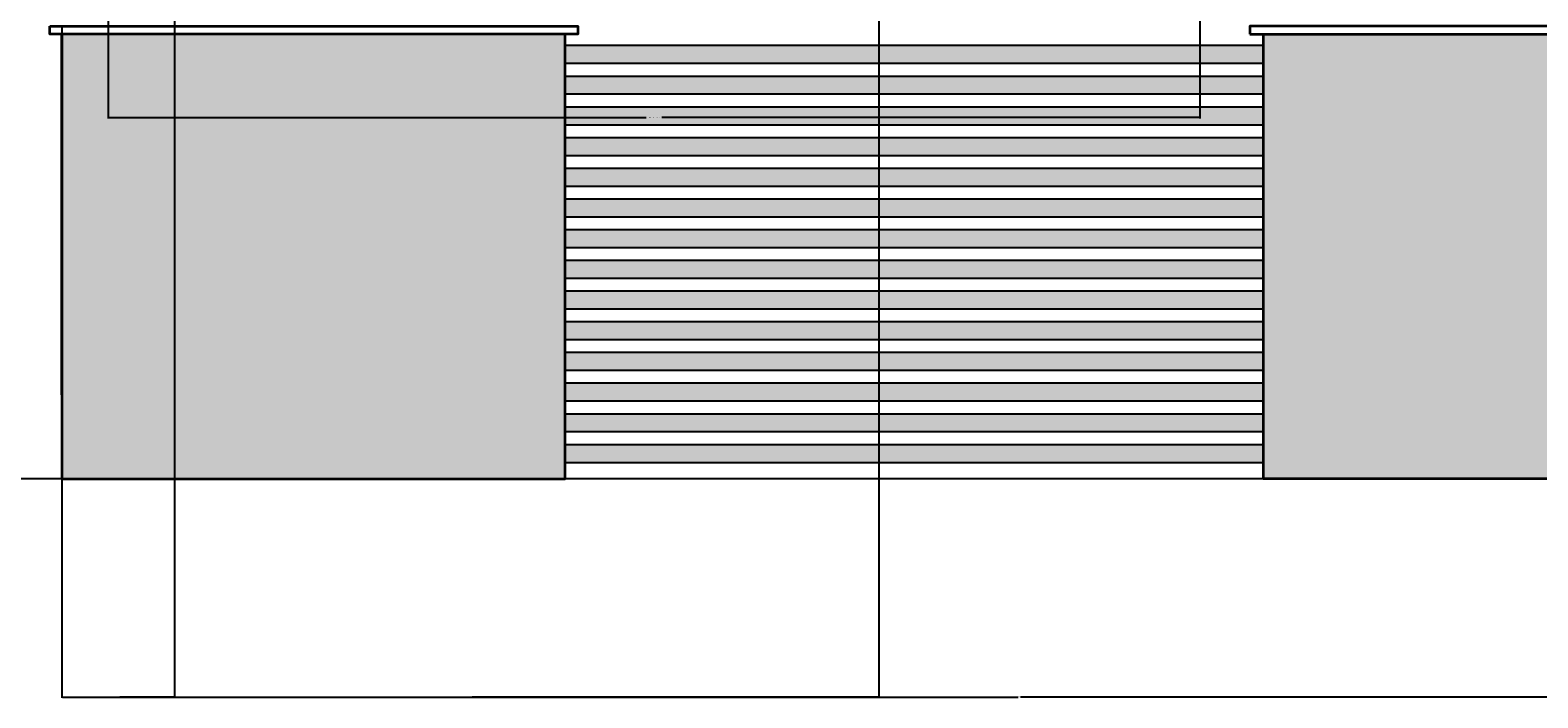
# Model space of a CAD drawing. Units: feet. Extents: x 1141 to 2858, y 751 to 1654.
# Tile 2 of 13: x 1718 to 2096, y 751 to 918. Entities that reach past the tile are written whole.
import ezdxf

# ---------------------------------------------------------------- set-up
doc = ezdxf.new("R2010")
doc.units = ezdxf.units.FT
for name, color, linetype, lineweight in [('A-ANNO-DIMS', 2, 'Continuous', 18), ('A-DOOR', 3, 'Continuous', 25), ('A-ELEV', 7, 'Continuous', 35), ('A-ELEV-PATT', 8, 'Continuous', 13)]:
    doc.layers.add(name, color=color, linetype=linetype, lineweight=lineweight)
doc.styles.get("Standard").update_dxf_attribs({"font": 'arial.ttf'})
doc.dimstyles.get("Standard").update_dxf_attribs({"dimtxt": 0.18, "dimasz": 0.18, "dimexe": 0.18, "dimexo": 0.0625, "dimgap": 0.09, "dimtad": 0, "dimtih": 1, "dimtoh": 1, "dimdec": 1, "dimzin": 0, "dimdsep": 46, "dimlunit": 3, "dimtxsty": 'Standard', "dimcen": 0.09, "dimadec": 0, "dimazin": 0, "dimtfac": 1, "dimtdec": 1, "dimtofl": 0, "dimtmove": 0, "dimatfit": 3, "dimfxl": 1, "dimtolj": 1, "dimtzin": 0, "dimarcsym": 0})

# ---------------------------------------------------------------- blocks, each defined once
blk = doc.blocks.new('*D18')
at = {"layer": 'A-ANNO-DIMS', "color": 0, "lineweight": -2, "transparency": 16777216}
for p, q in [((1737.61, 937.42), (1737.61, 896.25)), ((2011.29, 937.42), (2011.29, 896.25)), ((1737.79, 896.43), (1872.51, 896.43)), ((2011.11, 896.43), (1876.38, 896.43))]:
    blk.add_line(p, q, dxfattribs=at)
at = {"layer": 'A-ANNO-DIMS', "color": 0, "transparency": 16777216}
for points in [[(1737.79, 896.46), (1737.79, 896.4), (1737.61, 896.43)], [(2011.11, 896.46), (2011.11, 896.4), (2011.29, 896.43)]]:
    blk.add_solid(points, dxfattribs=at)
at = {"layer": 'Defpoints', "color": 0, "transparency": 16777216}
for p in [(1737.61, 937.48), (2011.29, 937.48), (2011.29, 896.43)]:
    blk.add_point(p, dxfattribs=at)
at = {"layer": 'A-ANNO-DIMS', "color": 0, "transparency": 16777216, "insert": (1874.45, 896.43), "char_height": 0.18, "attachment_point": 5}
blk.add_mtext('\\A1;BALCONY GLAZING A 274 TYP.', dxfattribs=at)
blk = doc.blocks.new('*D22')
at = {"layer": 'A-ANNO-DIMS', "color": 0, "lineweight": -2, "transparency": 16777216}
for p, q in [((1726.03, 805.84), (1726.03, 751.07)), ((2206.03, 805.84), (2206.03, 751.07)), ((1726.21, 751.25), (1965.74, 751.25)), ((2205.85, 751.25), (1966.32, 751.25))]:
    blk.add_line(p, q, dxfattribs=at)
at = {"layer": 'A-ANNO-DIMS', "color": 0, "transparency": 16777216}
for points in [[(1726.21, 751.28), (1726.21, 751.22), (1726.03, 751.25)], [(2205.85, 751.28), (2205.85, 751.22), (2206.03, 751.25)]]:
    blk.add_solid(points, dxfattribs=at)
at = {"layer": 'Defpoints', "color": 0, "transparency": 16777216}
for p in [(1726.03, 805.9), (2206.03, 805.9), (2206.03, 751.25)]:
    blk.add_point(p, dxfattribs=at)
at = {"layer": 'A-ANNO-DIMS', "color": 0, "transparency": 16777216, "insert": (1966.03, 751.25), "char_height": 0.18, "attachment_point": 5}
blk.add_mtext('\\A1;480', dxfattribs=at)
blk = doc.blocks.new('*D24')
at = {"layer": 'A-ANNO-DIMS', "color": 0, "lineweight": -2, "transparency": 16777216}
for p, q in [((1725.97, 1599.45), (1668.14, 1599.45)), ((1668.32, 1599.27), (1668.32, 1202.86)), ((1668.32, 806.08), (1668.32, 1202.49)), ((1725.97, 805.9), (1668.14, 805.9))]:
    blk.add_line(p, q, dxfattribs=at)
at = {"layer": 'A-ANNO-DIMS', "color": 0, "transparency": 16777216}
for points in [[(1668.29, 1599.27), (1668.35, 1599.27), (1668.32, 1599.45)], [(1668.29, 806.08), (1668.35, 806.08), (1668.32, 805.9)]]:
    blk.add_solid(points, dxfattribs=at)
at = {"layer": 'Defpoints', "color": 0, "transparency": 16777216}
for p in [(1668.32, 1599.45), (1726.03, 1599.45), (1726.03, 805.9)]:
    blk.add_point(p, dxfattribs=at)
at = {"layer": 'A-ANNO-DIMS', "color": 0, "transparency": 16777216, "insert": (1668.32, 1202.68), "char_height": 0.18, "attachment_point": 5}
blk.add_mtext('\\A1;793.6', dxfattribs=at)
blk = doc.blocks.new('*D39')
at = {"layer": 'A-ANNO-DIMS', "color": 0, "lineweight": -2, "transparency": 16777216}
for p, q in [((2319.24, 1599.45), (1668.14, 1599.45)), ((1668.32, 1599.27), (1668.32, 1202.86)), ((1668.32, 806.08), (1668.32, 1202.49)), ((2319.24, 805.9), (1668.14, 805.9))]:
    blk.add_line(p, q, dxfattribs=at)
at = {"layer": 'A-ANNO-DIMS', "color": 0, "transparency": 16777216}
for points in [[(1668.29, 1599.27), (1668.35, 1599.27), (1668.32, 1599.45)], [(1668.29, 806.08), (1668.35, 806.08), (1668.32, 805.9)]]:
    blk.add_solid(points, dxfattribs=at)
at = {"layer": 'Defpoints', "color": 0, "transparency": 16777216}
for p in [(1668.32, 1599.45), (2319.3, 1599.45), (2319.3, 805.9)]:
    blk.add_point(p, dxfattribs=at)
at = {"layer": 'A-ANNO-DIMS', "color": 0, "transparency": 16777216, "insert": (1668.32, 1202.68), "char_height": 0.18, "attachment_point": 5}
blk.add_mtext('\\A1;793.6', dxfattribs=at)
blk = doc.blocks.new('*D89')
at = {"layer": 'A-ANNO-DIMS', "color": 0, "lineweight": -2, "transparency": 16777216}
for p, q in [((1754.24, 946.71), (1754.24, 751.07)), ((1726.03, 919.28), (1726.03, 751.07)), ((1726.21, 751.25), (1739.76, 751.25)), ((1754.06, 751.25), (1740.52, 751.25))]:
    blk.add_line(p, q, dxfattribs=at)
at = {"layer": 'A-ANNO-DIMS', "color": 0, "transparency": 16777216}
for points in [[(1726.21, 751.28), (1726.21, 751.22), (1726.03, 751.25)], [(1754.06, 751.28), (1754.06, 751.22), (1754.24, 751.25)]]:
    blk.add_solid(points, dxfattribs=at)
at = {"layer": 'Defpoints', "color": 0, "transparency": 16777216}
for p in [(1754.24, 946.77), (1726.03, 919.34), (1754.24, 751.25)]:
    blk.add_point(p, dxfattribs=at)
at = {"layer": 'A-ANNO-DIMS', "color": 0, "transparency": 16777216, "insert": (1740.14, 751.25), "char_height": 0.18, "attachment_point": 5}
blk.add_mtext('\\A1;28.21', dxfattribs=at)
blk = doc.blocks.new('*D90')
at = {"layer": 'A-ANNO-DIMS', "color": 0, "lineweight": -2, "transparency": 16777216}
for p, q in [((1930.8, 951.37), (1930.8, 751.07)), ((1726.03, 919.28), (1726.03, 751.07)), ((1726.21, 751.25), (1827.95, 751.25)), ((1930.62, 751.25), (1828.88, 751.25))]:
    blk.add_line(p, q, dxfattribs=at)
at = {"layer": 'A-ANNO-DIMS', "color": 0, "transparency": 16777216}
for points in [[(1726.21, 751.28), (1726.21, 751.22), (1726.03, 751.25)], [(1930.62, 751.28), (1930.62, 751.22), (1930.8, 751.25)]]:
    blk.add_solid(points, dxfattribs=at)
at = {"layer": 'Defpoints', "color": 0, "transparency": 16777216}
for p in [(1930.8, 951.43), (1726.03, 919.34), (1930.8, 751.25)]:
    blk.add_point(p, dxfattribs=at)
at = {"layer": 'A-ANNO-DIMS', "color": 0, "transparency": 16777216, "insert": (1828.42, 751.25), "char_height": 0.18, "attachment_point": 5}
blk.add_mtext('\\A1;204.77', dxfattribs=at)

msp = doc.modelspace()

# ---------------------------------------------------------------- hatches: boundary and pattern name
at = {"layer": 'A-ELEV-PATT'}
h = msp.add_hatch(color=256, dxfattribs=at)
h.dxf.hatch_style = 1
h.paths.add_polyline_path([(2206.032, 1599.4527), (2192.689, 1599.4527), (2192.689, 919.339), (2206.032, 919.339)])
h.paths.add_polyline_path([(2190.2416, 1599.4527), (2175.463, 1599.4527), (2175.463, 919.339), (2190.2416, 919.339)])
h.paths.add_polyline_path([(2173.0156, 1599.4527), (2117.407, 1599.4527), (2117.407, 919.339), (2173.0156, 919.339)])
h.paths.add_polyline_path([(2022.8666, 1057.9008), (1726.032, 1057.9008), (1726.032, 925.9008), (2022.8666, 925.9008)])
h.paths.add_polyline_path([(1737.6123, 937.4811), (1737.6123, 1046.3205), (2011.2863, 1046.3205), (2011.2863, 937.4811)], flags=16)
h.paths.add_polyline_path([(1754.2423, 946.7736), (1754.2423, 1033.2183), (2004.2323, 1033.2183), (2004.2323, 946.7736), (2004.3069, 946.6754), (1906.0824, 946.6754)], flags=0)
h.paths.add_polyline_path([(1900.5421, 946.7736), (1857.5566, 946.7736), (1857.5566, 1033.2183), (1900.5421, 1033.2183)], flags=0)
h.paths.add_polyline_path([(1910.8368, 951.4297), (1910.8368, 1022.7957), (1999.478, 1022.7957), (1999.478, 951.4297)], flags=0)
h.paths.add_polyline_path([(1930.8039, 951.4297), (1930.8039, 1022.7957), (1932.373, 1022.7957), (1932.373, 951.4297)], flags=0)
h.paths.add_polyline_path([(1851.6414, 946.7736), (1826.5664, 946.7736), (1826.5664, 967.8234), (1793.4402, 967.8234), (1793.4402, 946.7736), (1790.4043, 946.7736), (1790.4043, 967.8234), (1754.2423, 967.8234), (1754.2423, 970.4796), (1790.4043, 970.4796), (1790.4043, 1033.2183), (1793.4402, 1033.2183), (1793.4402, 970.4796), (1826.5664, 970.4796), (1826.5664, 1033.2183), (1851.6414, 1033.2183)], flags=0)
h.paths.add_polyline_path([(1954.3728, 951.4297), (1954.3728, 1022.7957), (1955.9419, 1022.7957), (1955.9419, 951.4297)], flags=0)
h.paths.add_polyline_path([(1977.7327, 951.4297), (1977.7327, 1022.7957), (1979.3018, 1022.7957), (1979.3018, 951.4297)], flags=0)
h.paths.add_polyline_path([(2022.8666, 1193.2888), (1726.032, 1193.2888), (1726.032, 1061.2888), (2022.8666, 1061.2888)])
h.paths.add_polyline_path([(1737.6123, 1072.869), (1737.6123, 1181.7085), (2011.2863, 1181.7085), (2011.2863, 1072.869)], flags=16)
h.paths.add_polyline_path([(1754.2423, 1082.1616), (1754.2423, 1168.6063), (2004.2323, 1168.6063), (2004.2323, 1082.1616), (2004.3069, 1082.0634), (1906.0824, 1082.0634)], flags=0)
h.paths.add_polyline_path([(1900.5421, 1082.1616), (1857.5566, 1082.1616), (1857.5566, 1168.6063), (1900.5421, 1168.6063)], flags=0)
h.paths.add_polyline_path([(1910.8368, 1086.8177), (1910.8368, 1158.1837), (1999.478, 1158.1837), (1999.478, 1086.8177)], flags=0)
h.paths.add_polyline_path([(1930.8039, 1086.8177), (1930.8039, 1158.1837), (1932.373, 1158.1837), (1932.373, 1086.8177)], flags=0)
h.paths.add_polyline_path([(1851.6414, 1082.1616), (1826.5664, 1082.1616), (1826.5664, 1103.2114), (1793.4402, 1103.2114), (1793.4402, 1082.1616), (1790.4043, 1082.1616), (1790.4043, 1103.2114), (1754.2423, 1103.2114), (1754.2423, 1105.8676), (1790.4043, 1105.8676), (1790.4043, 1168.6063), (1793.4402, 1168.6063), (1793.4402, 1105.8676), (1826.5664, 1105.8676), (1826.5664, 1168.6063), (1851.6414, 1168.6063)], flags=0)
h.paths.add_polyline_path([(1954.3728, 1086.8177), (1954.3728, 1158.1837), (1955.9419, 1158.1837), (1955.9419, 1086.8177)], flags=0)
h.paths.add_polyline_path([(1977.7327, 1086.8177), (1977.7327, 1158.1837), (1979.3018, 1158.1837), (1979.3018, 1086.8177)], flags=0)
h.paths.add_polyline_path([(2022.8666, 1599.4527), (1726.032, 1599.4527), (1726.032, 1467.4527), (2022.8666, 1467.4527)])
h.paths.add_polyline_path([(2011.2863, 1479.033), (1737.6123, 1479.033), (1737.6123, 1587.8725), (2011.2863, 1587.8725)], flags=16)
h.paths.add_polyline_path([(2004.2323, 1488.3255), (1754.2423, 1488.3255), (1754.2423, 1574.7702), (2004.2323, 1574.7702)], flags=0)
h.paths.add_polyline_path([(1829.1345, 1544.6458), (1914.1177, 1544.6458), (1914.1177, 1539.5463), (1830.9097, 1539.5463), (1831.6817, 1537.3286), (1914.1177, 1537.3286), (1914.1177, 1532.2291), (1833.4569, 1532.2291), (1834.229, 1530.0113), (1914.1177, 1530.0113), (1914.1177, 1524.9118), (1836.0042, 1524.9118), (1836.7762, 1522.694), (1914.1177, 1522.694), (1914.1177, 1517.5946), (1838.5514, 1517.5946), (1839.3235, 1515.3768), (1914.1177, 1515.3768), (1914.1177, 1510.2773), (1841.0987, 1510.2773), (1841.8707, 1508.0595), (1914.1177, 1508.0595), (1914.1177, 1502.9601), (1843.6459, 1502.9601), (1844.4179, 1500.7423), (1914.1177, 1500.7423), (1914.1177, 1495.6428), (1846.1931, 1495.6428), (1846.9652, 1493.425), (1914.1177, 1493.425), (1914.1177, 1488.3255), (1848.6593, 1488.3255), (1848.6593, 1488.5583)], flags=0)
h.paths.add_polyline_path([(2117.407, 1464.0647), (1820.5724, 1464.0647), (1820.5724, 1332.0647), (2117.407, 1332.0647)])
h.paths.add_polyline_path([(2105.8267, 1452.4845), (2105.8267, 1343.645), (1832.1527, 1343.645), (1832.1527, 1452.4845)], flags=16)
h.paths.add_polyline_path([(2089.1967, 1439.3822), (2089.1967, 1352.9376), (1937.3566, 1352.9376), (1937.3566, 1352.8393), (1839.1321, 1352.8393), (1839.2067, 1352.9376), (1839.2067, 1439.3822), (1937.3566, 1439.3822)], flags=0)
h.paths.add_polyline_path([(2016.8727, 1439.3822), (2016.8727, 1376.6436), (2049.9988, 1376.6436), (2049.9988, 1439.3822), (2053.0347, 1439.3822), (2053.0347, 1376.6436), (2089.1967, 1376.6436), (2089.1967, 1373.9873), (2053.0347, 1373.9873), (2053.0347, 1352.9376), (2049.9988, 1352.9376), (2049.9988, 1373.9873), (2016.8727, 1373.9873), (2016.8727, 1352.9376), (1991.7976, 1352.9376), (1991.7976, 1439.3822)], flags=0)
h.paths.add_polyline_path([(1985.8824, 1439.3822), (1985.8824, 1352.9376), (1942.8969, 1352.9376), (1942.8969, 1439.3822)], flags=0)
h.paths.add_polyline_path([(1932.6022, 1428.9596), (1932.6022, 1357.5937), (1843.961, 1357.5937), (1843.961, 1428.9596)], flags=0)
h.paths.add_polyline_path([(1912.6351, 1428.9596), (1912.6351, 1357.5937), (1911.066, 1357.5937), (1911.066, 1428.9596)], flags=0)
h.paths.add_polyline_path([(1889.0662, 1428.9596), (1889.0662, 1357.5937), (1887.4971, 1357.5937), (1887.4971, 1428.9596)], flags=0)
h.paths.add_polyline_path([(1865.7063, 1428.9596), (1865.7063, 1357.5937), (1864.1372, 1357.5937), (1864.1372, 1428.9596)], flags=0)
h.paths.add_polyline_path([(2117.407, 1328.6768), (1820.5724, 1328.6768), (1820.5724, 1196.6768), (2117.407, 1196.6768)])
h.paths.add_polyline_path([(2105.8267, 1317.0965), (2105.8267, 1208.257), (1832.1527, 1208.257), (1832.1527, 1317.0965)], flags=16)
h.paths.add_polyline_path([(2089.1967, 1303.9943), (2089.1967, 1217.5496), (1937.3566, 1217.5496), (1937.3566, 1217.4513), (1839.1321, 1217.4513), (1839.2067, 1217.5496), (1839.2067, 1303.9943), (1937.3566, 1303.9943)], flags=0)
h.paths.add_polyline_path([(2016.8727, 1303.9943), (2016.8727, 1241.2556), (2049.9988, 1241.2556), (2049.9988, 1303.9943), (2053.0347, 1303.9943), (2053.0347, 1241.2556), (2089.1967, 1241.2556), (2089.1967, 1238.5993), (2053.0347, 1238.5993), (2053.0347, 1217.5496), (2049.9988, 1217.5496), (2049.9988, 1238.5993), (2016.8727, 1238.5993), (2016.8727, 1217.5496), (1991.7976, 1217.5496), (1991.7976, 1303.9943)], flags=0)
h.paths.add_polyline_path([(1985.8824, 1303.9943), (1985.8824, 1217.5496), (1942.8969, 1217.5496), (1942.8969, 1303.9943)], flags=0)
h.paths.add_polyline_path([(1932.6022, 1293.5716), (1932.6022, 1222.2057), (1843.961, 1222.2057), (1843.961, 1293.5716)], flags=0)
h.paths.add_polyline_path([(1912.6351, 1293.5716), (1912.6351, 1222.2057), (1911.066, 1222.2057), (1911.066, 1293.5716)], flags=0)
h.paths.add_polyline_path([(1889.0662, 1293.5716), (1889.0662, 1222.2057), (1887.4971, 1222.2057), (1887.4971, 1293.5716)], flags=0)
h.paths.add_polyline_path([(1865.7063, 1293.5716), (1865.7063, 1222.2057), (1864.1372, 1222.2057), (1864.1372, 1293.5716)], flags=0)
h.paths.add_polyline_path([(2206.032, 917.3598), (2027.2589, 917.3598), (2027.2589, 805.9008), (2206.032, 805.9008)])
h.paths.add_polyline_path([(1852.1771, 917.3598), (1726.032, 917.3598), (1726.032, 805.9008), (1852.1771, 805.9008)])
h.paths.add_polyline_path([(2063.3101, 1580.3829), (2093.938, 1580.3829), (2093.938, 1513.0494), (2063.3101, 1513.0494)])
h.paths.add_polyline_path([(2063.3101, 1580.3829), (2093.938, 1580.3829), (2093.938, 1513.0494), (2063.3101, 1513.0494)])
h = msp.add_hatch(color=256, dxfattribs=at)
h.dxf.hatch_style = 1
h.paths.add_polyline_path([(2004.2323, 1574.7702), (1754.2423, 1574.7702), (1763.3732, 1548.5407), (1979.2491, 1548.5407), (1979.2491, 1488.3255), (2004.2323, 1488.3255)])
h.paths.add_polyline_path([(1754.2423, 1574.7702), (1754.2423, 1488.3255), (1784.3349, 1488.3255)], flags=17)
h.paths.add_polyline_path([(1768.7403, 1548.5407), (1766.0183, 1548.5407), (1786.98, 1488.3255), (1789.702, 1488.3255)], flags=17)
h.paths.add_polyline_path([(1774.1074, 1548.5407), (1771.3854, 1548.5407), (1792.3471, 1488.3255), (1795.0692, 1488.3255)], flags=17)
h.paths.add_polyline_path([(1779.4746, 1548.5407), (1776.7525, 1548.5407), (1797.7142, 1488.3255), (1800.4363, 1488.3255)], flags=17)
h.paths.add_polyline_path([(1784.8417, 1548.5407), (1782.1197, 1548.5407), (1803.0814, 1488.3255), (1805.8034, 1488.3255)], flags=17)
h.paths.add_polyline_path([(1790.2088, 1548.5407), (1787.4868, 1548.5407), (1808.4485, 1488.3255), (1811.1705, 1488.3255)], flags=17)
h.paths.add_polyline_path([(1795.5759, 1548.5407), (1792.8539, 1548.5407), (1813.8156, 1488.3255), (1816.5376, 1488.3255)], flags=17)
h.paths.add_polyline_path([(1800.9431, 1548.5407), (1798.221, 1548.5407), (1819.1827, 1488.3255), (1821.9048, 1488.3255)], flags=17)
h.paths.add_polyline_path([(1806.3102, 1548.5407), (1803.5881, 1548.5407), (1824.5499, 1488.3255), (1827.2719, 1488.3255)], flags=17)
h.paths.add_polyline_path([(1811.6773, 1548.5407), (1808.9553, 1548.5407), (1829.917, 1488.3255), (1832.639, 1488.3255)], flags=17)
h.paths.add_polyline_path([(1817.0444, 1548.5407), (1814.3224, 1548.5407), (1835.2841, 1488.3255), (1838.0061, 1488.3255)], flags=17)
h.paths.add_polyline_path([(1822.4115, 1548.5407), (1819.6895, 1548.5407), (1840.6512, 1488.3255), (1843.3733, 1488.3255)], flags=17)
h.paths.add_polyline_path([(1827.7787, 1548.5407), (1825.0566, 1548.5407), (1846.0183, 1488.3255), (1848.6593, 1488.3255), (1848.6593, 1488.5583)], flags=17)
h.paths.add_polyline_path([(1914.1177, 1544.6458), (1829.1345, 1544.6458), (1830.9097, 1539.5463), (1914.1177, 1539.5463)], flags=17)
h.paths.add_polyline_path([(1914.1177, 1537.3286), (1831.6817, 1537.3286), (1833.4569, 1532.2291), (1914.1177, 1532.2291)], flags=17)
h.paths.add_polyline_path([(1914.1177, 1530.0113), (1834.229, 1530.0113), (1836.0042, 1524.9118), (1914.1177, 1524.9118)], flags=17)
h.paths.add_polyline_path([(1914.1177, 1522.694), (1836.7762, 1522.694), (1838.5514, 1517.5946), (1914.1177, 1517.5946)], flags=17)
h.paths.add_polyline_path([(1914.1177, 1515.3768), (1839.3235, 1515.3768), (1841.0987, 1510.2773), (1914.1177, 1510.2773)], flags=17)
h.paths.add_polyline_path([(1914.1177, 1508.0595), (1841.8707, 1508.0595), (1843.6459, 1502.9601), (1914.1177, 1502.9601)], flags=17)
h.paths.add_polyline_path([(1914.1177, 1500.7423), (1844.4179, 1500.7423), (1846.1931, 1495.6428), (1914.1177, 1495.6428)], flags=17)
h.paths.add_polyline_path([(1914.1177, 1493.425), (1846.9652, 1493.425), (1848.7404, 1488.3255), (1914.1177, 1488.3255)], flags=17)
h.paths.add_polyline_path([(1920.7331, 1548.5407), (1918.1624, 1548.5407), (1918.3509, 1488.3255), (1920.9216, 1488.3255)], flags=17)
h.paths.add_polyline_path([(1925.8019, 1548.5407), (1923.2312, 1548.5407), (1923.4197, 1488.3255), (1925.9904, 1488.3255)], flags=17)
h.paths.add_polyline_path([(1930.8708, 1548.5407), (1928.3, 1548.5407), (1928.4885, 1488.3255), (1931.0592, 1488.3255)], flags=17)
h.paths.add_polyline_path([(1935.9396, 1548.5407), (1933.3688, 1548.5407), (1933.5573, 1488.3255), (1936.128, 1488.3255)], flags=17)
h.paths.add_polyline_path([(1941.0084, 1548.5407), (1938.4376, 1548.5407), (1938.6261, 1488.3255), (1941.1968, 1488.3255)], flags=17)
h.paths.add_polyline_path([(1946.0772, 1548.5407), (1943.5064, 1548.5407), (1943.6949, 1488.3255), (1946.2656, 1488.3255)], flags=17)
h.paths.add_polyline_path([(1951.146, 1548.5407), (1948.5752, 1548.5407), (1948.7637, 1488.3255), (1951.3344, 1488.3255)], flags=17)
h.paths.add_polyline_path([(1956.2148, 1548.5407), (1953.644, 1548.5407), (1953.8325, 1488.3255), (1956.4032, 1488.3255)], flags=17)
h.paths.add_polyline_path([(1961.2836, 1548.5407), (1958.7128, 1548.5407), (1958.9013, 1488.3255), (1961.472, 1488.3255)], flags=17)
h.paths.add_polyline_path([(1966.3524, 1548.5407), (1963.7816, 1548.5407), (1963.9701, 1488.3255), (1966.5408, 1488.3255)], flags=17)
h.paths.add_polyline_path([(1971.4212, 1548.5407), (1968.8504, 1548.5407), (1969.0389, 1488.3255), (1971.6096, 1488.3255)], flags=17)
h.paths.add_polyline_path([(1976.49, 1548.5407), (1973.9192, 1548.5407), (1974.1077, 1488.3255), (1976.6784, 1488.3255)], flags=17)
h.paths.add_polyline_path([(2027.2589, 914.5568), (1852.1771, 914.5568), (1852.1771, 909.9657), (2027.2589, 909.9657)])
h.paths.add_polyline_path([(2027.2589, 906.8659), (1852.1771, 906.8659), (1852.1771, 902.2747), (2027.2589, 902.2747)])
h.paths.add_polyline_path([(2027.2589, 899.1749), (1852.1771, 899.1749), (1852.1771, 894.5837), (2027.2589, 894.5837)])
h.paths.add_polyline_path([(2027.2589, 891.4839), (1852.1771, 891.4839), (1852.1771, 886.8927), (2027.2589, 886.8927)])
h.paths.add_polyline_path([(2027.2589, 883.793), (1852.1771, 883.793), (1852.1771, 879.2018), (2027.2589, 879.2018)])
h.paths.add_polyline_path([(2027.2589, 876.102), (1852.1771, 876.102), (1852.1771, 871.5108), (2027.2589, 871.5108)])
h.paths.add_polyline_path([(2027.2589, 868.411), (1852.1771, 868.411), (1852.1771, 863.8198), (2027.2589, 863.8198)])
h.paths.add_polyline_path([(2027.2589, 860.72), (1852.1771, 860.72), (1852.1771, 856.1289), (2027.2589, 856.1289)])
h.paths.add_polyline_path([(2027.2589, 853.0291), (1852.1771, 853.0291), (1852.1771, 848.4379), (2027.2589, 848.4379)])
h.paths.add_polyline_path([(2027.2589, 845.3381), (1852.1771, 845.3381), (1852.1771, 840.7469), (2027.2589, 840.7469)])
h.paths.add_polyline_path([(2027.2589, 837.6471), (1852.1771, 837.6471), (1852.1771, 833.056), (2027.2589, 833.056)])
h.paths.add_polyline_path([(2027.2589, 829.9562), (1852.1771, 829.9562), (1852.1771, 825.365), (2027.2589, 825.365)])
h.paths.add_polyline_path([(2027.2589, 822.2652), (1852.1771, 822.2652), (1852.1771, 817.674), (2027.2589, 817.674)])
h.paths.add_polyline_path([(2027.2589, 814.5742), (1852.1771, 814.5742), (1852.1771, 809.983), (2027.2589, 809.983)])

# ---------------------------------------------------------------- linework, layer by layer
at = {"layer": 'A-DOOR'}
for points in [[(1852.1771, 914.5568), (2027.2589, 914.5568), (2027.2589, 909.9657), (1852.1771, 909.9657)], [(1852.1771, 914.5568), (2027.2589, 914.5568), (2027.2589, 909.9657), (1852.1771, 909.9657)], [(1852.1771, 906.8659), (2027.2589, 906.8659), (2027.2589, 902.2747), (1852.1771, 902.2747)], [(1852.1771, 906.8659), (2027.2589, 906.8659), (2027.2589, 902.2747), (1852.1771, 902.2747)], [(1852.1771, 899.1749), (2027.2589, 899.1749), (2027.2589, 894.5837), (1852.1771, 894.5837)], [(1852.1771, 899.1749), (2027.2589, 899.1749), (2027.2589, 894.5837), (1852.1771, 894.5837)], [(1852.1771, 891.4839), (2027.2589, 891.4839), (2027.2589, 886.8927), (1852.1771, 886.8927)], [(1852.1771, 891.4839), (2027.2589, 891.4839), (2027.2589, 886.8927), (1852.1771, 886.8927)], [(1852.1771, 883.793), (2027.2589, 883.793), (2027.2589, 879.2018), (1852.1771, 879.2018)], [(1852.1771, 883.793), (2027.2589, 883.793), (2027.2589, 879.2018), (1852.1771, 879.2018)], [(1852.1771, 876.102), (2027.2589, 876.102), (2027.2589, 871.5108), (1852.1771, 871.5108)], [(1852.1771, 876.102), (2027.2589, 876.102), (2027.2589, 871.5108), (1852.1771, 871.5108)], [(1852.1771, 868.411), (2027.2589, 868.411), (2027.2589, 863.8198), (1852.1771, 863.8198)], [(1852.1771, 868.411), (2027.2589, 868.411), (2027.2589, 863.8198), (1852.1771, 863.8198)], [(1852.1771, 860.72), (2027.2589, 860.72), (2027.2589, 856.1289), (1852.1771, 856.1289)], [(1852.1771, 860.72), (2027.2589, 860.72), (2027.2589, 856.1289), (1852.1771, 856.1289)], [(1852.1771, 853.0291), (2027.2589, 853.0291), (2027.2589, 848.4379), (1852.1771, 848.4379)], [(1852.1771, 853.0291), (2027.2589, 853.0291), (2027.2589, 848.4379), (1852.1771, 848.4379)], [(1852.1771, 845.3381), (2027.2589, 845.3381), (2027.2589, 840.7469), (1852.1771, 840.7469)], [(1852.1771, 845.3381), (2027.2589, 845.3381), (2027.2589, 840.7469), (1852.1771, 840.7469)], [(1852.1771, 837.6471), (2027.2589, 837.6471), (2027.2589, 833.056), (1852.1771, 833.056)], [(1852.1771, 837.6471), (2027.2589, 837.6471), (2027.2589, 833.056), (1852.1771, 833.056)], [(1852.1771, 829.9562), (2027.2589, 829.9562), (2027.2589, 825.365), (1852.1771, 825.365)], [(1852.1771, 829.9562), (2027.2589, 829.9562), (2027.2589, 825.365), (1852.1771, 825.365)], [(1852.1771, 822.2652), (2027.2589, 822.2652), (2027.2589, 817.674), (1852.1771, 817.674)], [(1852.1771, 822.2652), (2027.2589, 822.2652), (2027.2589, 817.674), (1852.1771, 817.674)], [(1852.1771, 814.5742), (2027.2589, 814.5742), (2027.2589, 809.983), (1852.1771, 809.983)], [(1852.1771, 814.5742), (2027.2589, 814.5742), (2027.2589, 809.983), (1852.1771, 809.983)]]:
    msp.add_lwpolyline(points, close=True, dxfattribs=at)
at = {"layer": 'A-ELEV'}
for p, q in [((1726.032, 827.009), (1726.032, 917.3598)), ((1726.032, 917.3598), (1726.032, 805.9008)), ((1726.032, 827.009), (1726.032, 917.3598)), ((1726.032, 917.3598), (1726.032, 805.9008))]:
    msp.add_line(p, q, dxfattribs=at)
for points in [[(1722.9707, 919.339), (1855.3916, 919.339), (1855.3916, 917.3598), (1722.9707, 917.3598)], [(1722.9707, 919.339), (1855.3916, 919.339), (1855.3916, 917.3598), (1722.9707, 917.3598)], [(2023.7788, 917.3598), (2209.7297, 917.3598), (2209.7297, 919.339), (2023.7788, 919.339)], [(2023.7788, 917.3598), (2209.7297, 917.3598), (2209.7297, 919.339), (2023.7788, 919.339)], [(1726.032, 805.9008), (1852.1771, 805.9008), (1852.1771, 917.3598), (1726.032, 917.3598)], [(1726.032, 805.9008), (1852.1771, 805.9008), (1852.1771, 917.3598), (1726.032, 917.3598)], [(2206.032, 805.9008), (2027.2589, 805.9008), (2027.2589, 917.3598), (2206.032, 917.3598)], [(2206.032, 805.9008), (2027.2589, 805.9008), (2027.2589, 917.3598), (2206.032, 917.3598)]]:
    msp.add_lwpolyline(points, close=True, dxfattribs=at)

# ---------------------------------------------------------------- dimensions: what is measured, and where the dimension line sits
at = {"layer": 'A-ANNO-DIMS'}
for p1, p2, picture in [((1726.032, 805.9008), (1726.032, 1599.4527), '*D24'), ((2319.3013, 805.9008), (2319.3013, 1599.4527), '*D39')]:
    dim = msp.add_linear_dim(base=(1668.3207, 1599.4527), p1=p1, p2=p2, angle=90, dimstyle='Standard', override={"dimdec": 1, "dimlfac": 1, "dimrnd": 0, "dimzin": 0, "dimdsep": 46, "dimlunit": 2}, dxfattribs=at)
    dim.commit()
    dim.dimension.update_dxf_attribs({"geometry": picture, "text_midpoint": (1668.3207, 1202.6768)})
for base, p1, p2, override, picture, middle in [((1930.8039, 751.2508), (1726.032, 919.339), (1930.8039, 951.4297), {"dimdec": 2, "dimlfac": 1, "dimrnd": 0, "dimzin": 0, "dimdsep": 46, "dimlunit": 2}, '*D90', (1828.418, 751.2508)), ((1754.2423, 751.2508), (1726.032, 919.339), (1754.2423, 946.7736), {"dimdec": 2, "dimlfac": 1, "dimrnd": 0, "dimzin": 0, "dimdsep": 46, "dimlunit": 2}, '*D89', (1740.1372, 751.2508)), ((2206.032, 751.2508), (1726.032, 805.9008), (2206.032, 805.9008), {"dimdec": 0, "dimlfac": 1, "dimrnd": 0, "dimzin": 0, "dimdsep": 46, "dimlunit": 2}, '*D22', (1966.032, 751.2508))]:
    dim = msp.add_linear_dim(base=base, p1=p1, p2=p2, dimstyle='Standard', override=override, dxfattribs=at)
    dim.commit()
    dim.dimension.update_dxf_attribs({"geometry": picture, "text_midpoint": middle})
dim = msp.add_linear_dim(base=(2011.2863, 896.43), p1=(1737.6123, 937.4811), p2=(2011.2863, 937.4811), text='BALCONY GLAZING A <> TYP.', dimstyle='Standard', override={"dimdec": 0, "dimlfac": 1, "dimrnd": 0, "dimzin": 0, "dimdsep": 46, "dimlunit": 2}, dxfattribs=at)
dim.commit()
dim.dimension.update_dxf_attribs({"geometry": '*D18', "text_midpoint": (1874.4493, 896.43)})

doc.saveas('drawing.dxf')
